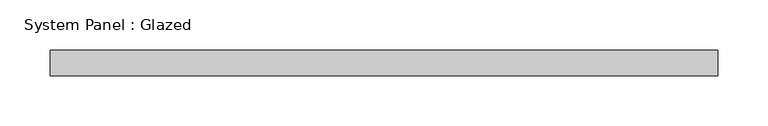
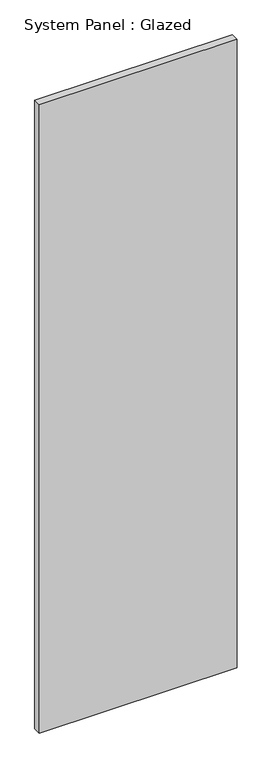
"""IFC4 building model written with IfcOpenShell, lengths in millimetres: plate geometry, System Panel : Glazed."""

from ifc_helpers import new_model, si_unit, origin, origin_with_axes, place, context, project, spatial, polyline, outline, extrude, source, transform, mapped, element, save


def system_panel_glazed_903d0225(model_context):
    return source(origin(), model_context, "Body", "SweptSolid", [
        extrude(outline(polyline([(333.375, 19.05), (-333.375, 19.05), (-333.375, 44.45), (333.375, 44.45), (333.375, 19.05)])), origin_with_axes(), (0.0, 0.0, 1.0), 2237.5663272),
    ])


if __name__ == "__main__":
    model = new_model("IFC4")
    model_context = context("Model", 3, world=origin())
    ifc_project = project(units=[si_unit("LENGTHUNIT", "METRE", prefix="MILLI")], contexts=[model_context])
    site = spatial("IfcSite", under=ifc_project)
    building = spatial("IfcBuilding", under=site)
    placement = place(None, origin())
    system_panel_glazed_shape = system_panel_glazed_903d0225(model_context)
    element("IfcPlate", 1, ObjectType="System Panel : Glazed", at=placement, inside=building, context=model_context, shape_type="MappedRepresentation", body=[
        mapped(system_panel_glazed_shape, transform((0.0, 0.0, 0.0), x_axis=(1.0, 0.0, 0.0), y_axis=(0.0, 1.0, 0.0), z_axis=(0.0, 0.0, 1.0))),
    ])
    save(model, "model.ifc")

# Revit data of these elements
# Type "System Panel : Glazed"
#   Construction Type Id = "GSP4R"
#   Analytic Construction = "1/8 in Pilkington single glazing"
#   Visual Light Transmittance = 0.9
#   Solar Heat Gain Coefficient = 0.86
#   Heat Transfer Coefficient (U) = 1.18115 BTU/(h·ft²·°F)
#   Define Thermal Properties by = 1
# Element 1 (IfcPlate, "System Panel : Glazed")
#   Materials on its faces: "Glass"
# Materials
#   "Glass": class "Glass", colour RGB 0 128 192, transparency 0.75, Description = "Soda Lime Glass", Cost = 0
